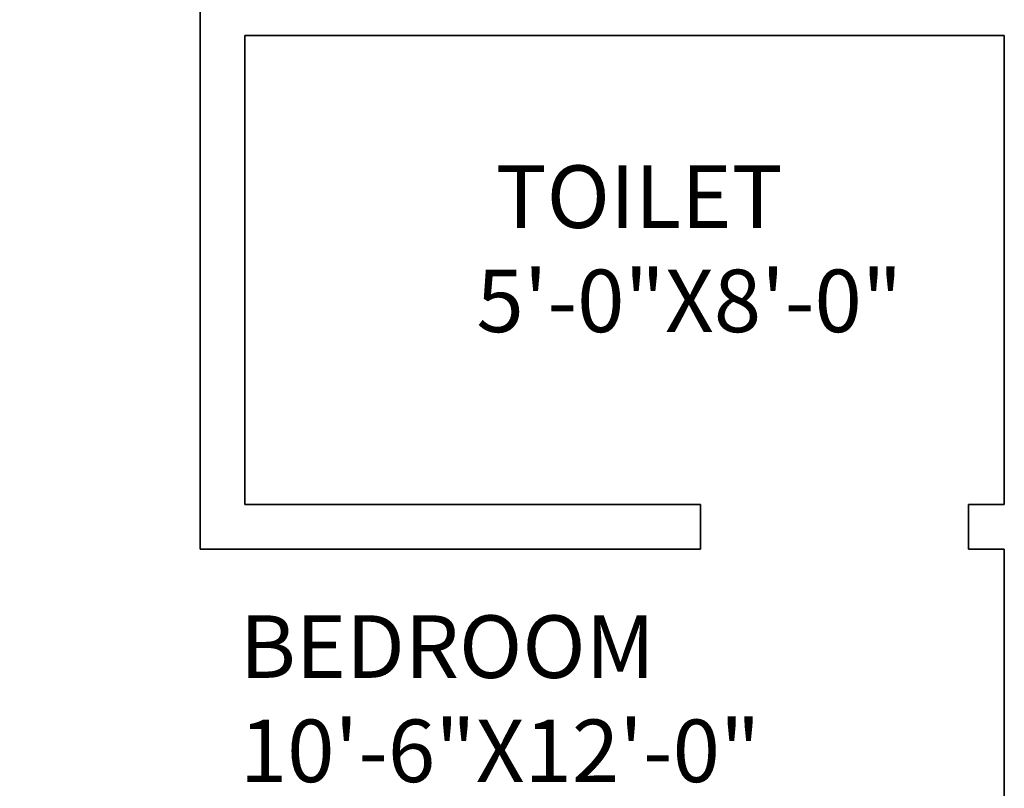
# Model space of a CAD drawing. Units: inches. Extents: x 3731 to 4318, y 1310 to 2388.
# Tile 47 of 57: x 4124 to 4234, y 2043 to 2129. Entities that reach past the tile are written whole.
import ezdxf

# ---------------------------------------------------------------- set-up
doc = ezdxf.new("R2010")
doc.units = ezdxf.units.IN
for name, color, linetype, lineweight in [('A-ANNO-DIMS', 2, 'Continuous', 18), ('A-AREA-IDEN', 7, 'Continuous', 18), ('A-WALL', 7, 'Continuous', 35)]:
    doc.layers.add(name, color=color, linetype=linetype, lineweight=lineweight)
doc.styles.get("Standard").update_dxf_attribs({"font": 'arial.ttf'})
doc.dimstyles.get("Standard").update_dxf_attribs({"dimtxt": 0.18, "dimasz": 0.18, "dimexe": 0.18, "dimexo": 0.0625, "dimgap": 0.09, "dimtad": 0, "dimtih": 1, "dimtoh": 1, "dimdec": 4, "dimzin": 0, "dimdsep": 46, "dimtxsty": 'Standard', "dimcen": 0.09, "dimadec": 0, "dimazin": 0, "dimtfac": 1, "dimtdec": 4, "dimtofl": 0, "dimtmove": 0, "dimatfit": 3, "dimfxl": 1, "dimtolj": 1, "dimtzin": 0, "dimarcsym": 0})

# ---------------------------------------------------------------- blocks, each defined once
blk = doc.blocks.new('*D38')
at = {"layer": 'A-ANNO-DIMS', "color": 0, "lineweight": -2, "transparency": 16777216}
for p, q in [((4103.27, 2262.38), (4318.34, 2262.38)), ((4318.16, 2262.2), (4318.16, 2103.06)), ((4318.16, 1943.56), (4318.16, 2102.7)), ((4234.27, 1943.38), (4318.34, 1943.38))]:
    blk.add_line(p, q, dxfattribs=at)
at = {"layer": 'A-ANNO-DIMS', "color": 0, "transparency": 16777216}
for points in [[(4318.13, 2262.2), (4318.19, 2262.2), (4318.16, 2262.38)], [(4318.13, 1943.56), (4318.19, 1943.56), (4318.16, 1943.38)]]:
    blk.add_solid(points, dxfattribs=at)
at = {"layer": 'Defpoints', "color": 0, "transparency": 16777216}
for p in [(4103.21, 2262.38), (4318.16, 2262.38), (4234.21, 1943.38)]:
    blk.add_point(p, dxfattribs=at)
at = {"layer": 'A-ANNO-DIMS', "color": 0, "transparency": 16777216, "insert": (4318.16, 2102.88), "char_height": 0.18, "attachment_point": 5}
blk.add_mtext('\\A1;319', dxfattribs=at)

msp = doc.modelspace()

# ---------------------------------------------------------------- linework, layer by layer
at = {"layer": 'A-WALL'}
for p, q in [((4144.21, 2189.38), (4144.21, 2069.38)), ((4234.21, 2126.88), (4149.21, 2126.88)), ((4149.21, 2126.88), (4149.21, 2074.38)), ((4234.21, 2126.88), (4234.21, 2074.38)), ((4149.21, 2074.38), (4200.21, 2074.38)), ((4200.21, 2074.38), (4200.21, 2069.38)), ((4230.21, 2074.38), (4230.21, 2069.38)), ((4230.21, 2074.38), (4234.21, 2074.38)), ((4144.21, 2069.38), (4200.21, 2069.38)), ((4230.21, 2069.38), (4234.21, 2069.38)), ((4234.21, 2069.38), (4234.21, 1943.38))]:
    msp.add_line(p, q, dxfattribs=at)

# ---------------------------------------------------------------- texts
at = {"layer": 'A-AREA-IDEN', "char_height": 7, "attachment_point": 1}
for s, insert in [(' TOILET\\P5\'-0"X8\'-0"', (4175.13, 2112.34)), ('BEDROOM\\P10\'-6"X12\'-0"', (4148.65, 2061.97))]:
    msp.add_mtext_dynamic_manual_height_columns(s, width=39.1687, gutter_width=12.5, heights=[0], dxfattribs=dict(at, insert=insert))

# ---------------------------------------------------------------- dimensions: what is measured, and where the dimension line sits
at = {"layer": 'A-ANNO-DIMS'}
dim = msp.add_linear_dim(base=(4318.16, 2262.38), p1=(4234.21, 1943.38), p2=(4103.21, 2262.38), angle=90, dimstyle='Standard', override={"dimdec": 0, "dimlfac": 1, "dimrnd": 0, "dimzin": 0, "dimdsep": 46, "dimlunit": 2}, dxfattribs=at)
dim.commit()
dim.dimension.update_dxf_attribs({"geometry": '*D38', "text_midpoint": (4318.16, 2102.88)})

doc.saveas('drawing.dxf')
